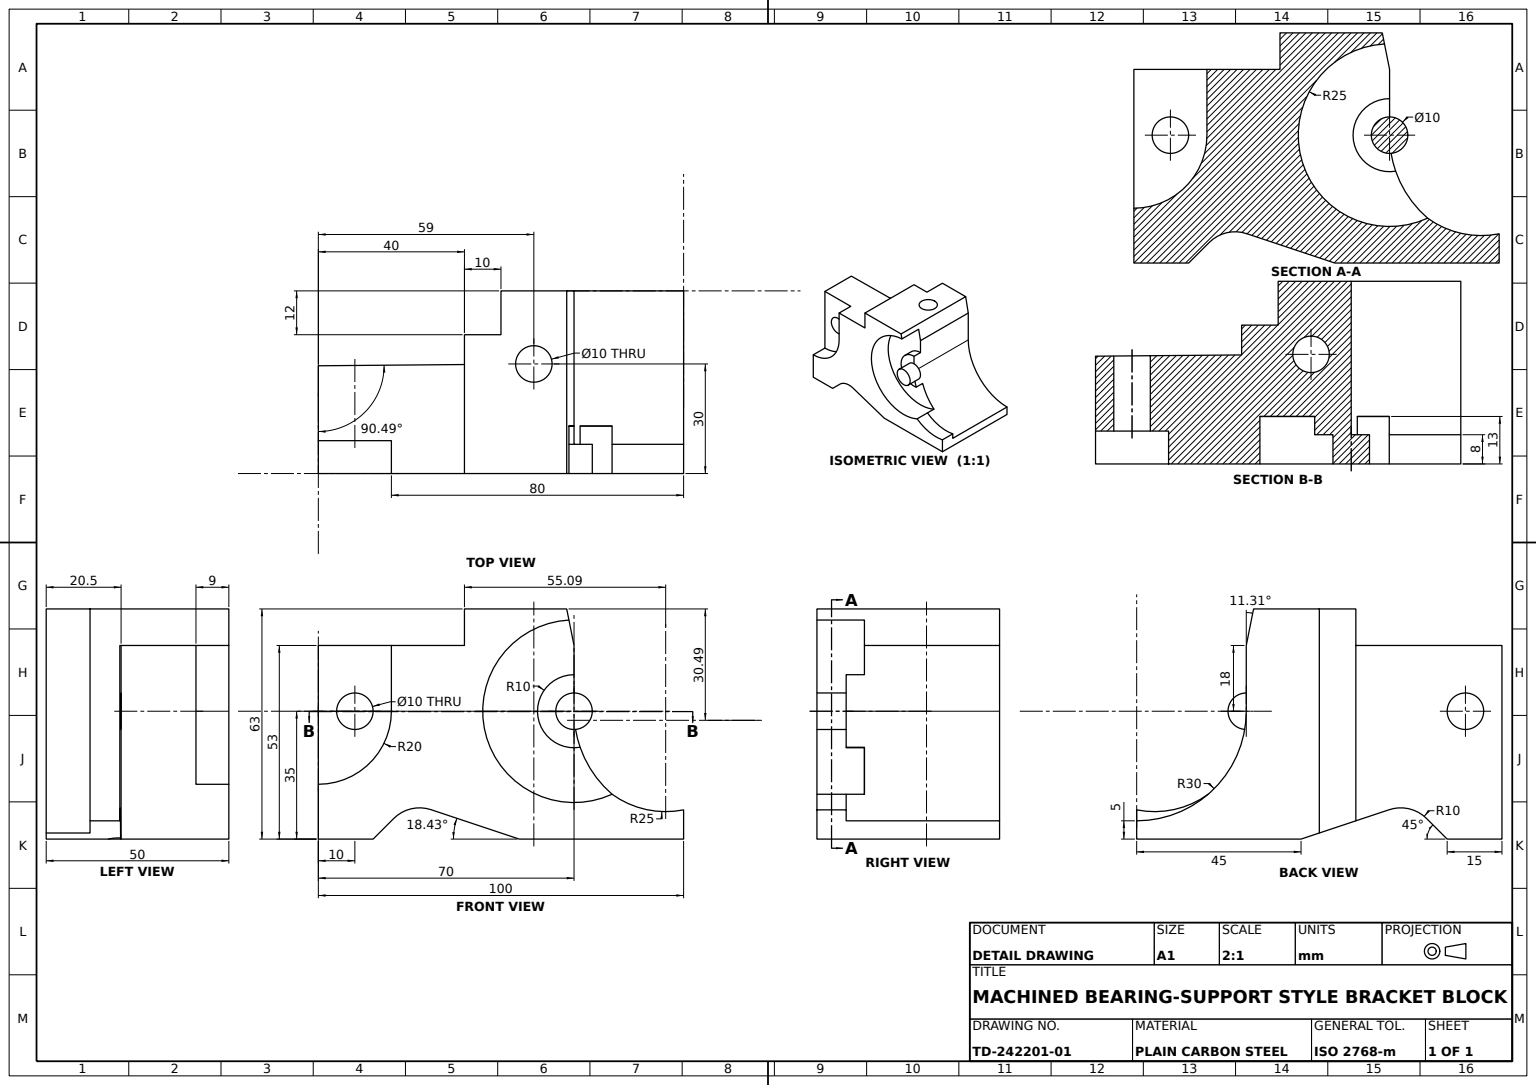
from build123d import *

# Parameters (mm, degrees)
BLOCK_BODY_DEPTH          = 50
BEARING_START             = -13
BEARING_ARC_RECESS_DEPTH  = 13
ARC_POCKET_SKETCH_R       = 10.03476875
ARC_POCKET_SKETCH_R_2     = 5
ARC_POCKET_DEPTH          = 8
PIN_10_SKETCH_R           = 5
PIN_10_DEPTH              = 8
SIDE_BOSS_DEPTH           = 8
PROFILE_RELIEF_CUT_DEPTH  = 129.33160172
STEP_CUT_DEPTH            = 9
STEP_NOTCH_DEPTH          = 126.099960032
SLOT_CUT_SKETCH_R         = 5
SLOT_CUT_DEPTH            = 129.33160172
TOP_RELIEF_CUT_DEPTH      = 129.33160172
TOP_RELIEF_CUT_DEPTH_BACK = 129.33160172
TOP_RELIEF_SKETCH_W       = 10
TOP_RELIEF_SKETCH_H       = 12


with BuildPart() as part:
    # Block Profile Sketch → Block Body (new body)
    with BuildSketch(Plane.XY):
        with BuildLine():
            ThreePointArc((70, 35), (78.786796564, 13.786796564), (100, 5))
            Line((100, 5), (100, 0))
            Line((100, 0), (0, 0))
            Line((0, 0), (0, 53))
            Line((0, 53), (40, 53))
            Line((40, 53), (40, 63))
            Line((40, 63), (50, 63))
            Line((50, 63), (68, 63))
            Line((68, 63), (70, 53))
            Line((70, 53), (70, 35))
        make_face()
    extrude(amount=BLOCK_BODY_DEPTH)

    # Bearing Arc Recess Sketch → Bearing Arc Recess (cut)
    with BuildSketch(Plane.XY.offset(50).offset(BEARING_START)):
        with BuildLine():
            ThreePointArc((80.416666667, 12.273516428), (91.040635288, 21.498456878), (95, 35))
            ThreePointArc((95, 35), (87.17838735, 53.163232313), (68.607759357, 59.961203216))
            Line((68.607759357, 59.961203216), (70, 53))
            Line((70, 53), (70, 45))
            ThreePointArc((70, 45), (77.071067812, 42.071067812), (80, 35))
            ThreePointArc((80, 35), (77.637626158, 28.545027756), (71.666666667, 25.139867028))
            ThreePointArc((71.666666667, 25.139867028), (75.192995333, 18.129537071), (80.416666667, 12.273516428))
        make_face()
        with BuildLine():
            Line((70, 53), (68.607759357, 59.961203216))
            ThreePointArc((68.607759357, 59.961203216), (45.732966105, 28.990751633), (80.416666667, 12.273516428))
            ThreePointArc((80.416666667, 12.273516428), (75.192995333, 18.129537071), (71.666666667, 25.139867028))
            ThreePointArc((71.666666667, 25.139867028), (60.035028105, 34.163737397), (70, 45))
            Line((70, 45), (70, 53))
        make_face()
    extrude(amount=BEARING_ARC_RECESS_DEPTH, mode=Mode.SUBTRACT)

    # Arc Pocket Sketch → Arc Pocket (cut)
    with BuildSketch(Plane.XY.offset(50)):
        with Locations((70, 35)):
            Circle(ARC_POCKET_SKETCH_R)
        with Locations((70, 35)):
            Circle(ARC_POCKET_SKETCH_R_2, mode=Mode.SUBTRACT)
    extrude(amount=-ARC_POCKET_DEPTH, mode=Mode.SUBTRACT)

    # Pin Ø10 Sketch → Pin Ø10 (add)
    with BuildSketch(Plane.XY.offset(50)):
        with Locations((70, 35)):
            Circle(PIN_10_SKETCH_R)
    extrude(amount=-PIN_10_DEPTH)

    # Side Boss Sketch → Side Boss (add)
    with BuildSketch(Plane.XY.offset(50)):
        with BuildLine():
            Line((80.416666667, 12.273516428), (80.416666667, 0))
            Line((80.416666667, 0), (100, 0))
            Line((100, 0), (100, 8))
            ThreePointArc((100, 8), (89.761290268, 8.088189193), (80.416666667, 12.273516428))
        make_face()
    extrude(amount=-SIDE_BOSS_DEPTH)

    # Profile Relief Sketch → Profile Relief Cut (cut, through all)
    with BuildSketch(Plane.XY.offset(50)):
        with BuildLine():
            Line((20.629839756, 5.629839756), (15, 0))
            Line((15, 0), (25, 0))
            Line((25, 0), (55, 0))
            Line((55, 0), (30.863185228, 8.045604924))
            ThreePointArc((30.863185228, 8.045604924), (25.403378362, 8.291261838), (20.629839756, 5.629839756))
        make_face()
    extrude(amount=-PROFILE_RELIEF_CUT_DEPTH, mode=Mode.SUBTRACT)

    # Step Cut Sketch → Step Cut (cut)
    with BuildSketch(Plane.XY.offset(50)):
        with BuildLine():
            Line((0, 35), (20, 35))
            ThreePointArc((20, 35), (16.946326412, 45.621771092), (8.717797887, 53))
            Line((8.717797887, 53), (0, 53))
            Line((0, 53), (0, 35))
        make_face()
        with BuildLine():
            ThreePointArc((8.717797887, 53), (16.946326412, 45.621771092), (20, 35))
            Line((20, 35), (20, 53))
            Line((20, 53), (8.717797887, 53))
        make_face()
        with BuildLine():
            ThreePointArc((0, 15), (14.142135624, 20.857864376), (20, 35))
            Line((20, 35), (0, 35))
            Line((0, 35), (0, 15))
        make_face()
    extrude(amount=-STEP_CUT_DEPTH, mode=Mode.SUBTRACT)

    # Step Notch Sketch → Step Notch (cut, through all)
    with BuildSketch(Plane.XY.offset(41)):
        with BuildLine():
            ThreePointArc((10, 40), (6.464466094, 31.464466094), (15, 35))
            Line((15, 35), (10, 35))
            Line((10, 35), (10, 40))
        make_face()
        with BuildLine():
            Line((10, 35), (15, 35))
            ThreePointArc((15, 35), (13.535533906, 38.535533906), (10, 40))
            Line((10, 40), (10, 35))
        make_face()
    extrude(amount=-STEP_NOTCH_DEPTH, mode=Mode.SUBTRACT)

    # Slot Cut Sketch → Slot Cut (cut, through all)
    with BuildSketch(Plane(origin=(0, 63, 0), x_dir=(1, 0, 0), z_dir=(0, 1, 0))):
        with Locations(Location((59, -20, 0), (0, 0, 270))):
            Circle(SLOT_CUT_SKETCH_R)
    extrude(amount=-SLOT_CUT_DEPTH, mode=Mode.SUBTRACT)

    # Top Relief Sketch → Top Relief Cut (cut, two sides: drawn at the far end of the back side and taken through both)
    with BuildSketch(Plane(origin=(0, 63, 0), x_dir=(1, 0, 0), z_dir=(0, 1, 0)).offset(-TOP_RELIEF_CUT_DEPTH_BACK)):
        with Locations((45, -6)):
            Rectangle(TOP_RELIEF_SKETCH_W, TOP_RELIEF_SKETCH_H)
        Polygon((40, -12), (40, 0), (0, 0), (0, -20.5), (40, -20.161016949), align=None)
    extrude(amount=TOP_RELIEF_CUT_DEPTH + TOP_RELIEF_CUT_DEPTH_BACK, mode=Mode.SUBTRACT)


solid = part.part
